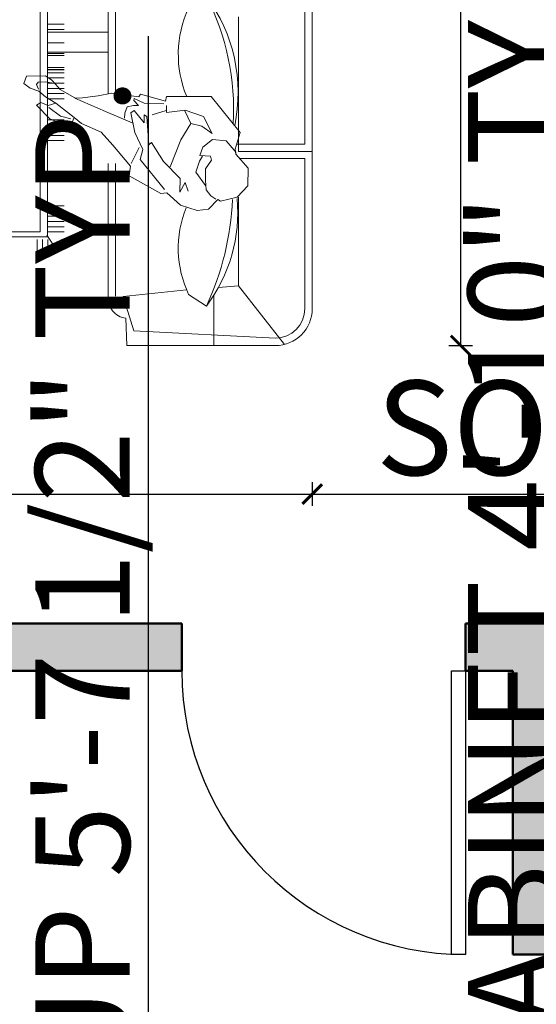
# Model space of a CAD drawing. Units: inches. Extents: x 375 to 1122, y 27 to 1069.
# Tile 74 of 155: x 601 to 667, y 667 to 792. Entities that reach past the tile are written whole.
import ezdxf

# ---------------------------------------------------------------- set-up
doc = ezdxf.new("R2010")
doc.units = ezdxf.units.IN
for name, color, linetype, lineweight in [('A-ANNO-DIMS', 2, 'Continuous', 18), ('A-WALL-PATT', 252, 'Continuous', 13), ('Doors', 150, 'Continuous', 25), ('Furniture', 30, 'Continuous', 18), ('Walls', 250, 'Continuous', 50)]:
    doc.layers.add(name, color=color, linetype=linetype, lineweight=lineweight)
doc.styles.get("Standard").update_dxf_attribs({"font": 'arial.ttf'})
doc.dimstyles.new('ISO-25', dxfattribs={"dimtxt": 12, "dimasz": 2.5, "dimexe": 1.5, "dimexo": 1.5, "dimtad": 1, "dimdec": 1, "dimlunit": 3, "dimtxsty": 'Standard', "dimblk": 'ARCHTICK', "dimcen": 2.5, "dimadec": 0, "dimazin": 0, "dimtfac": 1, "dimtdec": 1, "dimtmove": 0, "dimatfit": 3, "dimfxl": 1.5, "dimfxlon": 1, "dimarcsym": 0})

# ---------------------------------------------------------------- blocks, each defined once
blk = doc.blocks.new('*U8')
for p, q in [((-36, 0), (-36, 4)), ((0, 0), (0, 4))]:
    blk.add_line(p, q)
blk.add_lwpolyline([(0, 0), (0, -36), (-1.75, -36), (-1.75, 0)], close=True)
blk.add_arc((0, 0), 36, 180, 270)
blk = doc.blocks.new('*U12')
for p, q in [((0, 0), (0, -4)), ((24, 0), (24, -4))]:
    blk.add_line(p, q)
blk.add_lwpolyline([(0, 0), (0, 24), (1.75, 24), (1.75, 0)], close=True)
blk.add_arc((0, 0), 24, 0, 90)
blk = doc.blocks.new('A$C4DC51D13')
for p, q in [((3248.4, 487.7), (3248.4, 1772.3)), ((3215.6, 511), (3215.6, 1744.8)), ((4404, 1578.3), (4404, 904.6)), ((4437.5, 165.9), (4437.5, 1578.3)), ((3521.2, 1130.7), (3521.2, 1521.9)), ((3554.3, 1131.4), (3554.3, 1521.9)), ((4106.1, 1476.4), (4106.1, 872.1)), ((3248.8, 1443.4), (3322.7, 1443.4)), ((3248.8, 1419.9), (3322.7, 1419.9)), ((3250, 1407.8), (3519, 1407.8)), ((3248.8, 990.8), (3248.4, 1328.4)), ((3248.8, 1359), (3322.7, 1359)), ((3248.8, 1312.1), (3322.7, 1312.1)), ((3248.8, 1302.3), (3322.7, 1302.3)), ((3250, 1317.8), (3519, 1317.8)), ((3248.8, 1249), (3322.7, 1249)), ((3248.8, 1248.5), (3322.7, 1248.5)), ((3248.8, 1239.3), (3322.7, 1239.3)), ((3248.8, 1238.8), (3322.7, 1238.8)), ((3248.8, 1225.5), (3322.7, 1225.5)), ((3248.8, 1202.1), (3322.7, 1202.1)), ((3248.8, 1178.6), (3322.7, 1178.6)), ((3248.8, 1155.1), (3322.7, 1155.1)), ((3248.8, 1131.6), (3322.7, 1131.6)), ((3248.8, 1108.2), (3322.7, 1108.2)), ((3248.8, 1014.3), (3322.7, 1014.3)), ((3248.8, 990.8), (3322.7, 990.8)), ((3248.8, 967.3), (3322.7, 967.3)), ((3248.8, 943.8), (3322.7, 943.8)), ((3248.8, 920.4), (3322.7, 920.4)), ((4097.4, 904.6), (4404, 904.6)), ((4106.1, 871.5), (4437.5, 871.5)), ((4404, 840.7), (4110.5, 840.7)), ((4404, 165.9), (4404, 840.7)), ((3521.2, 816.9), (3521.2, 222.3)), ((3554.3, 816.9), (3554.3, 222.3)), ((4106.1, 267.8), (4106.1, 666.5)), ((3248.8, 627.8), (3322.7, 627.8)), ((3248.8, 604.4), (3322.7, 604.4)), ((3248.8, 580.9), (3322.7, 580.9)), ((3248.8, 557.4), (3322.7, 557.4)), ((3248.8, 533.9), (3322.7, 533.9)), ((1158.5, 487.7), (3248.4, 487.7)), ((3215.6, 511), (1196, 511)), ((3244.9, 495.1), (3290.3, 429)), ((3248.8, 510.5), (3322.7, 510.5)), ((3202.2, 476.3), (3202.2, 402.4)), ((3225.7, 476.3), (3225.7, 402.4)), ((3249.2, 476.3), (3249.2, 402.4)), ((4015.5, 260.8), (4106.1, 267.8)), ((4106.1, 267.8), (4312.2, 5.4)), ((3588, 220.6), (3873.1, 249.7)), ((3961.8, 177.4), (3882.1, 229.3)), ((3995.7, 0.4), (3995.7, 227)), ((3636.1, 66.6), (3588, 220.6)), ((3600.6, 122.5), (3605.1, 0.4)), ((4271.6, 33.5), (3636.1, 66.6)), ((3605.1, 0.4), (4271.6, 0.4))]:
    blk.add_line(p, q)
at = {"linetype": 'ByBlock'}
blk.add_lwpolyline([(3285.2, 1088.3), (3251.7, 1078.6), (3219, 1091.1), (3198.3, 1079.4), (3259.3, 1018.8), (3307.7, 998), (3330.8, 978), (3356, 995.1), (3367.5, 1023.6), (3401.2, 997.5), (3489.6, 958), (3542.4, 900.5), (3621.6, 805.3), (3615.5, 762.2), (3756.7, 683), (3783.9, 685.3), (3846.2, 629.9), (3920.9, 607.2), (3971.2, 612.7), (4013, 656), (4024.6, 648.7), (4100.1, 665.9), (4148.2, 716.6), (4149.9, 796.5), (4093.9, 859.3), (4090.7, 882.4), (4113.4, 957.1), (3983.4, 1118.2), (3782.9, 1118.2), (3777.7, 1097.2), (3665.2, 1129.2), (3657.9, 1117.6), (3537, 1133.7), (3476.2, 1121.9), (3393.3, 1110.9), (3371.2, 1111.9), (3304.9, 1150.4), (3283.7, 1173.4), (3267, 1191.9), (3239.5, 1211), (3154.4, 1209.5), (3142, 1176.8), (3171.1, 1155.3), (3209.3, 1142.5), (3238.9, 1117.5)], close=True, dxfattribs=at)
for points in [[(3207.2, 1152), (3198.7, 1171.9), (3206, 1183.5), (3237.5, 1184.7), (3284.8, 1177.6)], [(3629.1, 999.7), (3508, 1051.6), (3371, 1110.9)], [(3594.3, 1021.6), (3595.2, 1043.7), (3606.7, 1072.1), (3635, 1078.6), (3657, 1077.6), (3635.9, 1100.6), (3638, 1109.1), (3682.2, 1089.3), (3770.4, 1085.6)], [(3352.8, 1018.2), (3306.5, 1029.5), (3253.8, 1069.2)], [(3367.5, 1023.6), (3285.2, 1088.3)], [(3799.1, 802), (3846.8, 924.2), (3891.6, 998), (3942.1, 985.6), (3987.4, 952.2), (3948.2, 1028.7), (3866.1, 1057.7), (3783.2, 1046.8), (3782, 1078.3)], [(3879.5, 693.2), (3866.7, 732), (3842.7, 688.8), (3844.5, 750.8), (3769.6, 827.1), (3714.6, 911.9), (3703.1, 901.3), (3694, 1028.4), (3682.4, 1035.7), (3682.6, 1000), (3638.2, 1055.5), (3622.5, 1045.9), (3640.8, 956.7), (3675.9, 881.2), (3664.5, 834.9), (3774.4, 701)], [(3781.1, 1056.2), (3718.2, 1035.9)], [(3891.6, 998), (3865.1, 1053.5)], [(3624.7, 817.9), (3660.1, 889.6)], [(4096, 867.7), (4050.6, 918.9), (3989.6, 924.9), (3945.7, 891.1), (3932.2, 854.2), (3980.6, 851.3), (3984.9, 832.4), (3957.7, 794.4), (3958, 740.9), (3961.4, 699.9), (3981.4, 672.7), (4004.6, 658.1)], [(3957.1, 718.8), (3913.7, 778.5), (3930.3, 827.9), (3944.9, 851.1)]]:
    blk.add_lwpolyline(points, dxfattribs=at)
for centre, radius, start, end in [((3383, 1136.2), 721.4, 348.1046, 36.6442), ((2968.3, 1058.8), 1115.8, 356.7543, 27.0804), ((4324, 1306.8), 488.4, 154.7866, 202.7137), ((3404.4, 598.4), 698.5, 322.9389, 5.0789), ((2799, 717.9), 1282.3, 335.0725, 357.2152), ((4324, 437.4), 488.4, 158.2152, 205.2134), ((3610.6, 212), 90, 173.4179, 263.5749), ((4271.6, 165.9), 132.4, 270, 0), ((4271.6, 165.9), 165.9, 270, 0)]:
    blk.add_arc(centre, radius, start, end)
blk = doc.blocks.new('_ArchTick')
at = {"color": 0, "linetype": 'ByBlock', "const_width": 0.15}
blk.add_lwpolyline([(-0.5, -0.5), (0.5, 0.5)], dxfattribs=at)
blk = doc.blocks.new('*D43')
at = {"layer": 'A-ANNO-DIMS', "color": 0, "lineweight": -2, "transparency": 16777216}
for p, q in [((617.28, 580.53), (617.28, 790.11)), ((615.78, 580.53), (618.78, 580.53)), ((617.28, 513.06), (617.28, 580.53)), ((615.78, 513.06), (618.78, 513.06))]:
    blk.add_line(p, q, dxfattribs=at)
at = {"layer": 'Defpoints', "color": 0, "transparency": 16777216}
for p in [(607.16, 580.53), (617.28, 580.53), (607.16, 513.06)]:
    blk.add_point(p, dxfattribs=at)
at = {"layer": 'A-ANNO-DIMS', "color": 0, "lineweight": -2, "transparency": 16777216, "xscale": 2.5, "yscale": 2.5, "zscale": 2.5}
for p, rotation in [((617.28, 580.53), 90), ((617.28, 513.06), 270)]:
    blk.add_blockref('_ArchTick', p, dxfattribs=dict(at, rotation=rotation))
at = {"layer": 'A-ANNO-DIMS', "color": 0, "transparency": 16777216, "insert": (610.45, 686.57), "char_height": 12, "attachment_point": 5, "rotation": 90}
blk.add_mtext('BED GROUP 5\'-7 1/2" TYP.', dxfattribs=at)
blk = doc.blocks.new('*D45')
at = {"layer": 'A-ANNO-DIMS', "color": 0, "lineweight": -2, "transparency": 16777216}
for p, q in [((697.69, 641.67), (697.69, 644.67)), ((722.01, 641.67), (722.01, 644.67)), ((697.69, 643.17), (559.76, 643.17)), ((722.01, 643.17), (697.69, 643.17))]:
    blk.add_line(p, q, dxfattribs=at)
at = {"layer": 'Defpoints', "color": 0, "transparency": 16777216}
for p in [(697.69, 643.17), (697.69, 639.53), (722.01, 639.53)]:
    blk.add_point(p, dxfattribs=at)
at = {"layer": 'A-ANNO-DIMS', "color": 0, "lineweight": -2, "transparency": 16777216, "xscale": 2.5, "yscale": 2.5, "zscale": 2.5, "rotation": 180}
blk.add_blockref('_ArchTick', (697.69, 643.17), dxfattribs=at)
at = {"layer": 'A-ANNO-DIMS', "color": 0, "lineweight": -2, "transparency": 16777216, "xscale": 2.5, "yscale": 2.5, "zscale": 2.5}
blk.add_blockref('_ArchTick', (722.01, 643.17), dxfattribs=at)
at = {"layer": 'A-ANNO-DIMS', "color": 0, "transparency": 16777216, "insert": (627.47, 650), "char_height": 12, "attachment_point": 5}
blk.add_mtext('WC 2\'-0 1/2" TYP.', dxfattribs=at)
blk = doc.blocks.new('*D57')
at = {"layer": 'A-ANNO-DIMS', "color": 0, "lineweight": -2, "transparency": 16777216}
for p, q in [((512.46, 733.49), (512.46, 730.49)), ((638.07, 733.49), (638.07, 730.49)), ((512.46, 731.99), (638.07, 731.99)), ((638.07, 731.99), (839.76, 731.99))]:
    blk.add_line(p, q, dxfattribs=at)
at = {"layer": 'Defpoints', "color": 0, "transparency": 16777216}
for p in [(512.46, 750.84), (638.07, 750.84), (638.07, 731.99)]:
    blk.add_point(p, dxfattribs=at)
at = {"layer": 'A-ANNO-DIMS', "color": 0, "lineweight": -2, "transparency": 16777216, "xscale": 2.5, "yscale": 2.5, "zscale": 2.5, "rotation": 180}
blk.add_blockref('_ArchTick', (512.46, 731.99), dxfattribs=at)
at = {"layer": 'A-ANNO-DIMS', "color": 0, "lineweight": -2, "transparency": 16777216, "xscale": 2.5, "yscale": 2.5, "zscale": 2.5}
blk.add_blockref('_ArchTick', (638.07, 731.99), dxfattribs=at)
at = {"layer": 'A-ANNO-DIMS', "color": 0, "transparency": 16777216, "insert": (740.16, 738.83), "char_height": 12, "attachment_point": 5}
blk.add_mtext('SOFA SET 10\'-5 1/2" TYP.', dxfattribs=at)
blk = doc.blocks.new('*D58')
at = {"layer": 'A-ANNO-DIMS', "color": 0, "lineweight": -2, "transparency": 16777216}
for p, q in [((656.91, 835.53), (656.91, 940.29)), ((655.41, 835.53), (658.41, 835.53)), ((656.91, 750.84), (656.91, 835.53)), ((655.41, 750.84), (658.41, 750.84))]:
    blk.add_line(p, q, dxfattribs=at)
at = {"layer": 'Defpoints', "color": 0, "transparency": 16777216}
for p in [(638.07, 835.53), (656.91, 835.53), (638.07, 750.84)]:
    blk.add_point(p, dxfattribs=at)
at = {"layer": 'A-ANNO-DIMS', "color": 0, "lineweight": -2, "transparency": 16777216, "xscale": 2.5, "yscale": 2.5, "zscale": 2.5}
for p, rotation in [((656.91, 835.53), 90), ((656.91, 750.84), 270)]:
    blk.add_blockref('_ArchTick', p, dxfattribs=dict(at, rotation=rotation))
at = {"layer": 'A-ANNO-DIMS', "color": 0, "transparency": 16777216, "insert": (650.08, 889.16), "char_height": 12, "attachment_point": 5, "rotation": 90}
blk.add_mtext('7\'-0 1/2" TYP.', dxfattribs=at)
blk = doc.blocks.new('*D79')
at = {"layer": 'A-ANNO-DIMS', "color": 0, "lineweight": -2, "transparency": 16777216}
for p, q in [((672.21, 647.53), (672.21, 810.92)), ((670.71, 647.53), (673.71, 647.53)), ((672.21, 589.53), (672.21, 647.53)), ((670.71, 589.53), (673.71, 589.53))]:
    blk.add_line(p, q, dxfattribs=at)
at = {"layer": 'Defpoints', "color": 0, "transparency": 16777216}
for p in [(663.51, 647.53), (672.21, 647.53), (663.51, 589.53)]:
    blk.add_point(p, dxfattribs=at)
at = {"layer": 'A-ANNO-DIMS', "color": 0, "lineweight": -2, "transparency": 16777216, "xscale": 2.5, "yscale": 2.5, "zscale": 2.5}
for p, rotation in [((672.21, 647.53), 90), ((672.21, 589.53), 270)]:
    blk.add_blockref('_ArchTick', p, dxfattribs=dict(at, rotation=rotation))
at = {"layer": 'A-ANNO-DIMS', "color": 0, "transparency": 16777216, "insert": (665.38, 730.47), "char_height": 12, "attachment_point": 5, "rotation": 90}
blk.add_mtext('CABINET 4\'-10" TYP.', dxfattribs=at)
blk = doc.blocks.new('*D82')
at = {"layer": 'A-ANNO-DIMS', "color": 0, "lineweight": -2, "transparency": 16777216}
for p, q in [((401.51, 1009.53), (398.51, 1009.53)), ((400.01, 160.53), (400.01, 1009.53)), ((401.51, 160.53), (398.51, 160.53))]:
    blk.add_line(p, q, dxfattribs=at)
at = {"layer": 'Defpoints', "color": 0, "transparency": 16777216}
for p in [(400.01, 1009.53), (630.53, 1009.53), (630.53, 160.53)]:
    blk.add_point(p, dxfattribs=at)
at = {"layer": 'A-ANNO-DIMS', "color": 0, "lineweight": -2, "transparency": 16777216, "xscale": 2.5, "yscale": 2.5, "zscale": 2.5}
for p, rotation in [((400.01, 1009.53), 90), ((400.01, 160.53), 270)]:
    blk.add_blockref('_ArchTick', p, dxfattribs=dict(at, rotation=rotation))
at = {"layer": 'A-ANNO-DIMS', "color": 0, "transparency": 16777216, "insert": (393.26, 585.03), "char_height": 12, "attachment_point": 5, "rotation": 90}
blk.add_mtext('70\'-9"', dxfattribs=at)
blk = doc.blocks.new('*D92')
at = {"layer": 'A-ANNO-DIMS', "color": 0, "lineweight": -2, "transparency": 16777216}
for p, q in [((621.51, 1052.53), (621.51, 1055.53)), ((657.51, 1052.53), (657.51, 1055.53)), ((621.51, 1054.03), (657.51, 1054.03))]:
    blk.add_line(p, q, dxfattribs=at)
at = {"layer": 'Defpoints', "color": 0, "transparency": 16777216}
for p in [(657.51, 1054.03), (621.51, 460.53), (657.51, 460.53)]:
    blk.add_point(p, dxfattribs=at)
at = {"layer": 'A-ANNO-DIMS', "color": 0, "lineweight": -2, "transparency": 16777216, "xscale": 2.5, "yscale": 2.5, "zscale": 2.5, "rotation": 180}
blk.add_blockref('_ArchTick', (621.51, 1054.03), dxfattribs=at)
at = {"layer": 'A-ANNO-DIMS', "color": 0, "lineweight": -2, "transparency": 16777216, "xscale": 2.5, "yscale": 2.5, "zscale": 2.5}
blk.add_blockref('_ArchTick', (657.51, 1054.03), dxfattribs=at)
at = {"layer": 'A-ANNO-DIMS', "color": 0, "transparency": 16777216, "insert": (639.51, 1060.78), "char_height": 12, "attachment_point": 5}
blk.add_mtext('3\'-0"', dxfattribs=at)
blk = doc.blocks.new('*D93')
at = {"layer": 'A-ANNO-DIMS', "color": 0, "lineweight": -2, "transparency": 16777216}
for p, q in [((400.01, 673.53), (400.01, 709.38)), ((401.51, 673.53), (398.51, 673.53)), ((400.01, 649.53), (400.01, 673.53)), ((401.51, 649.53), (398.51, 649.53))]:
    blk.add_line(p, q, dxfattribs=at)
at = {"layer": 'Defpoints', "color": 0, "transparency": 16777216}
for p in [(400.01, 673.53), (663.51, 673.53), (663.51, 649.53)]:
    blk.add_point(p, dxfattribs=at)
at = {"layer": 'A-ANNO-DIMS', "color": 0, "lineweight": -2, "transparency": 16777216, "xscale": 2.5, "yscale": 2.5, "zscale": 2.5}
for p, rotation in [((400.01, 673.53), 90), ((400.01, 649.53), 270)]:
    blk.add_blockref('_ArchTick', p, dxfattribs=dict(at, rotation=rotation))
at = {"layer": 'A-ANNO-DIMS', "color": 0, "transparency": 16777216, "insert": (393.26, 692.7), "char_height": 12, "attachment_point": 5, "rotation": 90}
blk.add_mtext('2\'-0"', dxfattribs=at)

msp = doc.modelspace()

# ---------------------------------------------------------------- hatches: boundary and pattern name
at = {"layer": 'A-WALL-PATT'}
h = msp.add_hatch(color=256, dxfattribs=at)
h.dxf.hatch_style = 1
h.paths.add_polyline_path([(962.01, 388.53), (989.01, 388.53), (989.01, 394.53), (962.01, 394.53), (932.01, 394.53), (932.01, 397.53), (923.01, 397.53), (923.01, 394.53), (842.01, 394.53), (842.01, 334.53), (839.51, 334.53), (839.51, 328.53), (854.01, 328.53), (854.01, 334.53), (848.01, 334.53), (848.01, 388.53), (953.01, 388.53), (953.01, 356.08), (962.01, 356.08), (962.01, 358.55), (989.01, 358.55), (989.01, 364.55), (962.01, 364.55)])
h.paths.add_polyline_path([(989.01, 502.53), (932.01, 502.53), (932.01, 583.53), (932.01, 593.53), (923.01, 593.53), (923.01, 583.53), (854.01, 583.53), (854.01, 556.53), (863.01, 556.53), (863.01, 574.53), (923.01, 574.53), (923.01, 502.53), (863.01, 502.53), (863.01, 520.53), (854.01, 520.53), (854.01, 502.53), (773.01, 502.53), (773.01, 493.53), (788.01, 493.53), (788.01, 402.03), (722.01, 402.03), (722.01, 373.53), (728.01, 373.53), (728.01, 396.03), (788.01, 396.03), (788.01, 373.53), (794.01, 373.53), (794.01, 430.53), (814.01, 430.53), (814.01, 436.53), (794.01, 436.53), (794.01, 493.53), (923.01, 493.53), (923.01, 487.53), (932.01, 487.53), (932.01, 493.53), (983.01, 493.53), (983.01, 473.53), (989.01, 473.53)])
h.paths.add_polyline_path([(797.01, 325.53), (805.01, 325.53), (805.01, 328.53), (807.51, 328.53), (807.51, 334.53), (791.01, 334.53), (791.01, 226.53), (770.76, 226.53), (770.76, 217.53), (791.01, 217.53), (791.01, 187.53), (855.01, 187.53), (855.01, 196.53), (797.01, 196.53)])
h.paths.add_polyline_path([(989.01, 238.53), (962.01, 238.53), (962.01, 256.42), (953.01, 256.42), (953.01, 229.53), (980.01, 229.53), (980.01, 196.53), (915.01, 196.53), (915.01, 187.53), (989.01, 187.53)])
h.paths.add_polyline_path([(962.01, 334.53), (884.01, 334.53), (884.01, 328.53), (918.01, 328.53), (918.01, 325.53), (932.01, 325.53), (932.01, 328.53), (953.01, 328.53), (953.01, 304.42), (962.01, 304.42)])
h.paths.add_polyline_path([(606.51, 283.53), (609.51, 283.53), (609.51, 289.53), (600.51, 289.53), (600.51, 196.53), (578.51, 196.53), (578.51, 187.53), (606.51, 187.53), (606.51, 196.53)])
h.paths.add_polyline_path([(666.51, 292.53), (660.51, 292.53), (660.51, 289.53), (633.51, 289.53), (633.51, 283.53), (660.51, 283.53), (660.51, 196.53), (628.01, 196.53), (628.01, 187.53), (630.53, 187.53), (630.53, 160.53), (636.53, 160.53), (636.53, 187.53), (660.51, 187.53), (660.51, 160.53), (666.51, 160.53), (666.51, 217.53), (686.76, 217.53), (686.76, 226.53), (666.51, 226.53)])
h.paths.add_polyline_path([(480.51, 256.42), (471.51, 256.42), (471.51, 238.53), (444.51, 238.53), (444.51, 187.53), (518.51, 187.53), (518.51, 196.53), (453.51, 196.53), (453.51, 229.53), (480.51, 229.53)])
h.paths.add_polyline_path([(480.51, 328.53), (652.51, 328.53), (652.51, 325.53), (660.51, 325.53), (660.51, 322.53), (666.51, 322.53), (666.51, 334.53), (507.51, 334.53), (507.51, 360.53), (498.51, 360.53), (498.51, 334.53), (471.51, 334.53), (471.51, 304.42), (480.51, 304.42)])
h.paths.add_polyline_path([(507.51, 484.53), (498.51, 484.53), (498.51, 444.53), (507.51, 444.53), (507.51, 454.53), (621.51, 454.53), (621.51, 460.53), (507.51, 460.53)])
h.paths.add_polyline_path([(672.51, 604.53), (683.26, 604.53), (683.26, 613.53), (669.51, 613.53), (669.51, 649.53), (663.51, 649.53), (663.51, 589.53), (507.51, 589.53), (507.51, 613.53), (498.51, 613.53), (498.51, 556.53), (507.51, 556.53), (507.51, 580.53), (663.51, 580.53), (663.51, 520.53), (669.51, 520.53), (669.51, 556.53), (683.26, 556.53), (683.26, 565.53), (672.51, 565.53)])
h.paths.add_polyline_path([(731.01, 667.53), (734.01, 667.53), (734.01, 676.53), (728.01, 676.53), (728.01, 715.53), (657.51, 715.53), (657.51, 709.53), (663.51, 709.53), (663.51, 673.53), (669.51, 673.53), (669.51, 709.53), (722.01, 709.53), (722.01, 613.53), (704.76, 613.53), (704.76, 604.53), (722.01, 604.53), (722.01, 565.53), (704.76, 565.53), (704.76, 556.53), (722.01, 556.53), (722.01, 502.53), (722.01, 460.53), (669.51, 460.53), (669.51, 496.53), (663.51, 496.53), (663.51, 460.53), (657.51, 460.53), (657.51, 454.53), (728.01, 454.53), (728.01, 493.53), (734.01, 493.53), (734.01, 502.53), (731.01, 502.53)])
h.paths.add_polyline_path([(986.01, 718.53), (959.01, 718.53), (959.01, 727.53), (950.01, 727.53), (950.01, 709.53), (977.01, 709.53), (977.01, 676.53), (794.01, 676.53), (794.01, 805.53), (802.01, 805.53), (802.01, 808.53), (804.51, 808.53), (804.51, 814.53), (788.01, 814.53), (788.01, 774.03), (728.01, 774.03), (728.01, 796.53), (722.01, 796.53), (722.01, 768.03), (788.01, 768.03), (788.01, 676.53), (773.01, 676.53), (773.01, 667.53), (923.01, 667.53), (923.01, 657.53), (932.01, 657.53), (932.01, 667.53), (986.01, 667.53)])
h.paths.add_polyline_path([(621.51, 715.53), (507.51, 715.53), (507.51, 733.53), (498.51, 733.53), (498.51, 715.53), (498.51, 685.53), (507.51, 685.53), (507.51, 709.53), (621.51, 709.53)])
h.paths.add_polyline_path([(666.51, 847.03), (660.51, 847.03), (660.51, 844.53), (652.51, 844.53), (652.51, 841.53), (480.51, 841.53), (480.51, 859.53), (471.51, 859.53), (471.51, 835.53), (498.51, 835.53), (498.51, 817.53), (507.51, 817.53), (507.51, 835.53), (666.51, 835.53)])
h.paths.add_polyline_path([(480.51, 940.53), (453.51, 940.53), (453.51, 973.53), (518.51, 973.53), (518.51, 982.53), (444.51, 982.53), (444.51, 931.53), (471.51, 931.53), (471.51, 907.53), (480.51, 907.53)])
h.paths.add_polyline_path([(606.51, 982.53), (578.51, 982.53), (578.51, 973.53), (600.51, 973.53), (600.51, 880.53), (609.51, 880.53), (609.51, 886.53), (606.51, 886.53)])
h.paths.add_polyline_path([(666.51, 943.53), (686.76, 943.53), (686.76, 952.53), (666.51, 952.53), (666.51, 1009.53), (660.51, 1009.53), (660.51, 982.53), (636.53, 982.53), (636.53, 1009.53), (630.53, 1009.53), (630.53, 982.53), (628.01, 982.53), (628.01, 973.53), (660.51, 973.53), (660.51, 886.53), (633.51, 886.53), (633.51, 880.53), (660.51, 880.53), (660.51, 877.03), (666.51, 877.03)])
h.paths.add_polyline_path([(986.01, 874.53), (932.01, 874.53), (932.01, 877.53), (923.01, 877.53), (923.01, 874.53), (788.01, 874.53), (788.01, 868.53), (788.01, 844.53), (794.01, 844.53), (794.01, 868.53), (839.01, 868.53), (839.01, 814.53), (836.51, 814.53), (836.51, 808.53), (851.01, 808.53), (851.01, 814.53), (845.01, 814.53), (845.01, 868.53), (986.01, 868.53)])
h.paths.add_polyline_path([(959.01, 838.55), (986.01, 838.55), (986.01, 844.55), (959.01, 844.55), (959.01, 847.03), (950.01, 847.03), (950.01, 814.53), (881.01, 814.53), (881.01, 808.53), (918.01, 808.53), (918.01, 805.53), (932.01, 805.53), (932.01, 808.53), (950.01, 808.53), (950.01, 793.53), (959.01, 793.53)])
h.paths.add_polyline_path([(986.01, 982.53), (899.01, 982.53), (899.01, 973.53), (923.01, 973.53), (923.01, 967.53), (932.01, 967.53), (932.01, 973.53), (980.01, 973.53), (980.01, 953.53), (986.01, 953.53)])
h.paths.add_polyline_path([(851.01, 982.53), (788.01, 982.53), (788.01, 952.53), (770.76, 952.53), (770.76, 943.53), (788.01, 943.53), (788.01, 910.53), (814.01, 910.53), (814.01, 916.53), (794.01, 916.53), (794.01, 973.53), (851.01, 973.53)])

# ---------------------------------------------------------------- linework, layer by layer
at = {"layer": 'Walls'}
for p, q in [((507.51, 715.53), (621.51, 715.53)), ((621.51, 709.53), (621.51, 715.53)), ((657.51, 709.53), (657.51, 715.53)), ((657.51, 715.53), (728.01, 715.53)), ((507.51, 709.53), (621.51, 709.53)), ((657.51, 709.53), (663.51, 709.53)), ((663.51, 673.53), (663.51, 709.53)), ((669.51, 673.53), (663.51, 673.53))]:
    msp.add_line(p, q, dxfattribs=at)

# ---------------------------------------------------------------- block references
at = {"layer": 'Doors'}
msp.add_blockref('*U8', (657.51, 709.53), dxfattribs=at)
at = {"layer": 'Doors', "rotation": 270}
msp.add_blockref('*U12', (669.51, 673.53), dxfattribs=at)
at = {"layer": 'Furniture', "xscale": 0.0282665567793757, "yscale": 0.0282665567793757, "zscale": 0.0282665567793757}
msp.add_blockref('A$C4DC51D13', (512.64, 750.84), dxfattribs=at)

# ---------------------------------------------------------------- dimensions: what is measured, and where the dimension line sits
at = {"layer": 'A-ANNO-DIMS'}
dim = msp.add_linear_dim(base=(657.51, 1054.03), p1=(621.51, 460.53), p2=(657.51, 460.53), dimstyle='ISO-25', override={"dimdec": 1, "dimlfac": 1, "dimrnd": 0, "dimzin": 1, "dimdsep": 46, "dimlunit": 4, "dimfrac": 2}, dxfattribs=at)
dim.commit()
dim.dimension.update_dxf_attribs({"geometry": '*D92', "text_midpoint": (639.51, 1060.78)})
for base, p1, p2, picture, middle in [((400.01, 1009.53), (630.53, 160.53), (630.53, 1009.53), '*D82', (393.26, 585.03)), ((400.01, 673.53), (663.51, 649.53), (663.51, 673.53), '*D93', (393.26, 692.7))]:
    dim = msp.add_linear_dim(base=base, p1=p1, p2=p2, angle=90, dimstyle='ISO-25', override={"dimdec": 1, "dimlfac": 1, "dimrnd": 0, "dimzin": 1, "dimdsep": 46, "dimlunit": 4, "dimfrac": 2}, dxfattribs=at)
    dim.commit()
    dim.dimension.update_dxf_attribs({"geometry": picture, "text_midpoint": middle})
for base, p1, p2, angle, text, picture, middle in [((656.91, 835.53), (638.07, 750.84), (638.07, 835.53), 90, '<> TYP.', '*D58', (650.08, 889.16)), ((672.21, 647.53), (663.51, 589.53), (663.51, 647.53), 90, 'CABINET <> TYP.', '*D79', (665.38, 730.47)), ((617.28, 580.53), (607.16, 513.06), (607.16, 580.53), 90, 'BED GROUP <> TYP.', '*D43', (610.45, 686.57)), ((697.69, 643.17), (722.01, 639.53), (697.69, 639.53), 180, 'WC <> TYP.', '*D45', (627.47, 650))]:
    dim = msp.add_linear_dim(base=base, p1=p1, p2=p2, angle=angle, text=text, dimstyle='ISO-25', override={"dimdec": 1, "dimlfac": 1, "dimrnd": 0, "dimzin": 1, "dimdsep": 46, "dimlunit": 4, "dimfrac": 2}, dxfattribs=at)
    dim.commit()
    dim.dimension.update_dxf_attribs({"geometry": picture, "text_midpoint": middle})
dim = msp.add_linear_dim(base=(638.07, 731.99), p1=(512.46, 750.84), p2=(638.07, 750.84), text='SOFA SET <> TYP.', dimstyle='ISO-25', override={"dimdec": 1, "dimlfac": 1, "dimrnd": 0, "dimzin": 1, "dimdsep": 46, "dimlunit": 4, "dimfrac": 2}, dxfattribs=at)
dim.commit()
dim.dimension.update_dxf_attribs({"geometry": '*D57', "text_midpoint": (740.16, 738.83)})

doc.saveas('drawing.dxf')
